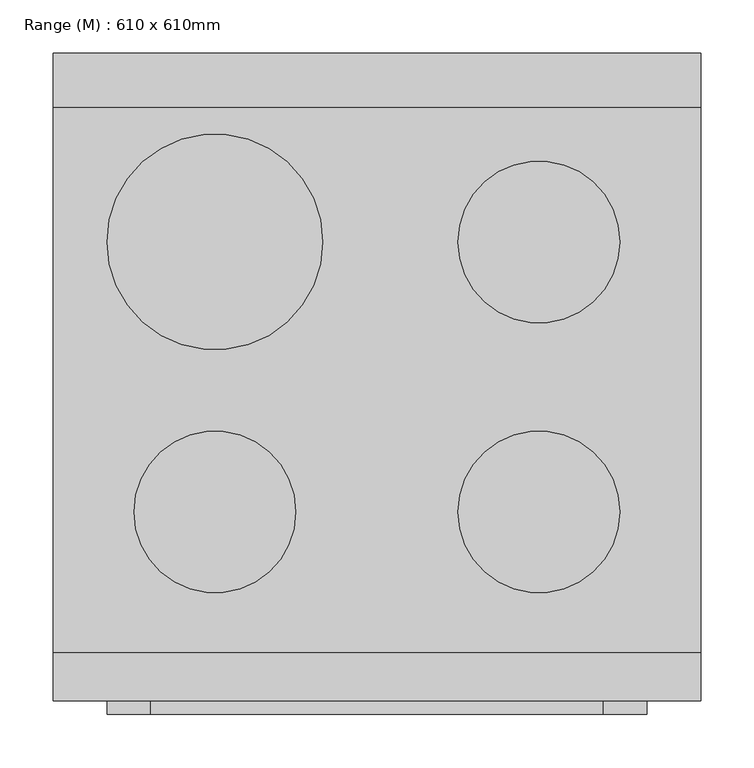
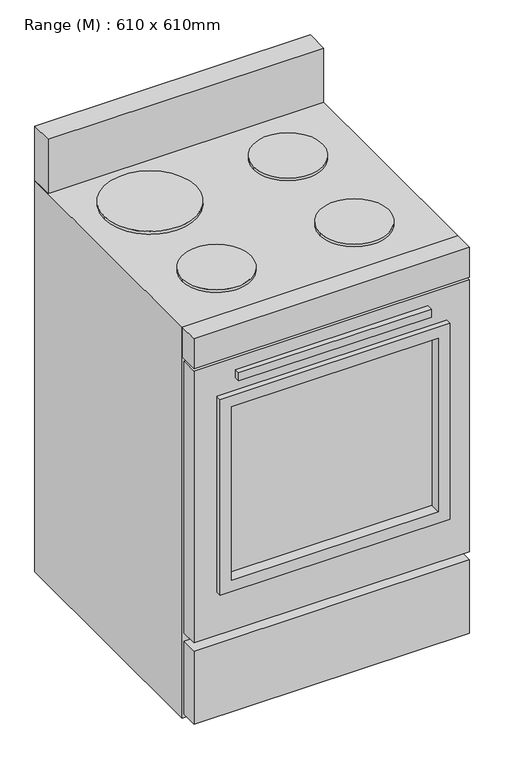
"""IFC4 building model written with IfcOpenShell, lengths in millimetres: proxy geometry, Range (M) : 610 x 610mm."""

from ifc_helpers import new_model, si_unit, point, frame, frame_2d, origin, place, context, project, spatial, polyline, circle_curve, trimmed, segment, composite_curve, outline, extrude, source, transform, mapped, element, save


def range_m_610_x_610mm_88bdc8d1(model_context):
    return source(origin(), model_context, "Body", "SweptSolid", [
        extrude(outline(polyline([(517.925, -12.7), (91.687309, -12.7), (91.687309, 0.0), (517.925, 0.0), (517.925, -12.7)])), frame((0.0, 0.0, 791.2768639), z_axis=(0.0, 0.0, 1.0), x_axis=(1.0, 0.0, 0.0)), (0.0, 0.0, 1.0), 19.05),
        extrude(outline(polyline([(533.8, 12.7), (76.2, 12.7), (76.2, 19.05), (533.8, 19.05), (533.8, 12.7)])), frame((0.0, 0.0, 330.2), z_axis=(0.0, 0.0, 1.0), x_axis=(1.0, 0.0, 0.0)), (0.0, 0.0, 1.0), 406.4),
        extrude(outline(polyline([(610.0, 0.0), (0.0, 0.0), (0.0, 45.0), (610.0, 45.0), (610.0, 0.0)])), frame((0.0, 0.0, 844.7720355), z_axis=(0.0, 0.0, 1.0), x_axis=(1.0, 0.0, 0.0)), (0.0, 0.0, 1.0), 69.6279645),
        extrude(outline(polyline([(762.0, 559.2), (762.0, 50.8), (304.8, 50.8), (304.8, 559.2), (762.0, 559.2)]), holes=[polyline([(736.6, 533.8), (330.2, 533.8), (330.2, 76.2), (736.6, 76.2), (736.6, 533.8)])]), frame((0.0, -12.7, 0.0), z_axis=(0.0, 1.0, 0.0), x_axis=(0.0, 0.0, 1.0)), (0.0, 0.0, 1.0), 38.1),
        extrude(outline(composite_curve([segment(trimmed(circle_curve(frame_2d((152.4, 432.2)), 101.6), [point((50.8, 432.2))], [point((254.0, 432.2))], False, "CARTESIAN"), True, "CONTINUOUS"), segment(trimmed(circle_curve(frame_2d((152.4, 432.2)), 101.6), [point((254.0, 432.2))], [point((50.8, 432.2))], False, "CARTESIAN"), True, "CONTINUOUS")], self_intersect=False)), frame((0.0, 0.0, 914.4), z_axis=(0.0, 0.0, 1.0), x_axis=(1.0, 0.0, 0.0)), (0.0, 0.0, 1.0), 6.35),
        extrude(outline(composite_curve([segment(trimmed(circle_curve(frame_2d((457.6, 432.2)), 76.2), [point((381.4, 432.2))], [point((533.8, 432.2))], False, "CARTESIAN"), True, "CONTINUOUS"), segment(trimmed(circle_curve(frame_2d((457.6, 432.2)), 76.2), [point((533.8, 432.2))], [point((381.4, 432.2))], False, "CARTESIAN"), True, "CONTINUOUS")], self_intersect=False)), frame((0.0, 0.0, 914.4), z_axis=(0.0, 0.0, 1.0), x_axis=(1.0, 0.0, 0.0)), (0.0, 0.0, 1.0), 6.35),
        extrude(outline(composite_curve([segment(trimmed(circle_curve(frame_2d((457.6, 177.8)), 76.2), [point((381.4, 177.8))], [point((533.8, 177.8))], False, "CARTESIAN"), True, "CONTINUOUS"), segment(trimmed(circle_curve(frame_2d((457.6, 177.8)), 76.2), [point((533.8, 177.8))], [point((381.4, 177.8))], False, "CARTESIAN"), True, "CONTINUOUS")], self_intersect=False)), frame((0.0, 0.0, 914.4), z_axis=(0.0, 0.0, 1.0), x_axis=(1.0, 0.0, 0.0)), (0.0, 0.0, 1.0), 6.35),
        extrude(outline(composite_curve([segment(trimmed(circle_curve(frame_2d((152.4, 177.8)), 76.2), [point((76.2, 177.8))], [point((228.6, 177.8))], False, "CARTESIAN"), True, "CONTINUOUS"), segment(trimmed(circle_curve(frame_2d((152.4, 177.8)), 76.2), [point((228.6, 177.8))], [point((76.2, 177.8))], False, "CARTESIAN"), True, "CONTINUOUS")], self_intersect=False)), frame((0.0, 0.0, 914.4), z_axis=(0.0, 0.0, 1.0), x_axis=(1.0, 0.0, 0.0)), (0.0, 0.0, 1.0), 6.35),
        extrude(outline(polyline([(25.4, 610.0), (584.6, 610.0), (584.6, 584.6), (25.4, 584.6), (25.4, 610.0)])), frame((0.0, 0.0, 254.0), z_axis=(0.0, 0.0, 1.0), x_axis=(1.0, 0.0, 0.0)), (0.0, 0.0, 1.0), 635.2220355),
        extrude(outline(polyline([(838.4220355, 610.0), (838.4220355, 0.0), (203.2, 0.0), (203.2, 610.0), (838.4220355, 610.0)]), holes=[polyline([(762.0, 559.2), (304.8, 559.2), (304.8, 50.8), (762.0, 50.8), (762.0, 559.2)])]), frame((0.0, 0.0, 0.0), z_axis=(0.0, 1.0, 0.0), x_axis=(0.0, 0.0, 1.0)), (0.0, 0.0, 1.0), 38.1),
        extrude(outline(polyline([(610.0, 0.0), (0.0, 0.0), (0.0, 38.1), (610.0, 38.1), (610.0, 0.0)])), frame((0.0, 0.0, 12.7), z_axis=(0.0, 0.0, 1.0), x_axis=(1.0, 0.0, 0.0)), (0.0, 0.0, 1.0), 171.45),
        extrude(outline(polyline([(914.4, 610.0), (914.4, 0.0), (0.0, 0.0), (0.0, 610.0), (914.4, 610.0)]), holes=[polyline([(889.2220355, 584.6), (254.0, 584.6), (254.0, 25.4), (889.2220355, 25.4), (889.2220355, 584.6)])]), frame((0.0, 45.0, 0.0), z_axis=(0.0, 1.0, 0.0), x_axis=(0.0, 0.0, 1.0)), (0.0, 0.0, 1.0), 565.0),
        extrude(outline(polyline([(610.0, 610.0), (610.0, 559.2), (0.0, 559.2), (0.0, 610.0), (610.0, 610.0)])), frame((0.0, 0.0, 914.4), z_axis=(0.0, 0.0, 1.0), x_axis=(1.0, 0.0, 0.0)), (0.0, 0.0, 1.0), 127.0),
    ])


if __name__ == "__main__":
    model = new_model("IFC4")
    model_context = context("Model", 3, world=origin())
    ifc_project = project(units=[si_unit("LENGTHUNIT", "METRE", prefix="MILLI")], contexts=[model_context])
    site = spatial("IfcSite", under=ifc_project)
    building = spatial("IfcBuilding", under=site)
    placement = place(None, origin())
    range_m_610_x_610mm_shape = range_m_610_x_610mm_88bdc8d1(model_context)
    element("IfcBuildingElementProxy", 1, Name="Range (M) : 610 x 610mm", ObjectType="Range (M) : 610 x 610mm", at=placement, inside=building, context=model_context, shape_type="MappedRepresentation", body=[
        mapped(range_m_610_x_610mm_shape, transform((0.0, 0.0, 0.0), x_axis=(1.0, 0.0, 0.0), y_axis=(0.0, 1.0, 0.0), z_axis=(0.0, 0.0, 1.0))),
    ])
    save(model, "model.ifc")

# Revit data of these elements
# Type "Range (M) : 610 x 610mm"
#   Depth = 2' - 0.01575"
#   Width = 2' - 0.01575"
#   Burner Material = Metal - Chrome
#   Range Material = Metal - Painted Finish - Ivory,Matte
#   Default Elevation = 0
#   Assembly Code = ""
# Element 1 (IfcBuildingElementProxy, "Range (M) : 610 x 610mm")
#   Materials on its faces: "Metal - Painted Finish - Ivory,Matte", "Metal - Chrome", "Glass"
# Materials
#   "Metal - Chrome": colour RGB 17 17 17, transparency 0
#   "Metal - Painted Finish - Ivory,Matte": colour RGB 247 247 239, transparency 0
#   "Glass": class "Glass", colour RGB 0 128 192, transparency 0.75, Description = "Soda Lime Glass", Cost = 0
